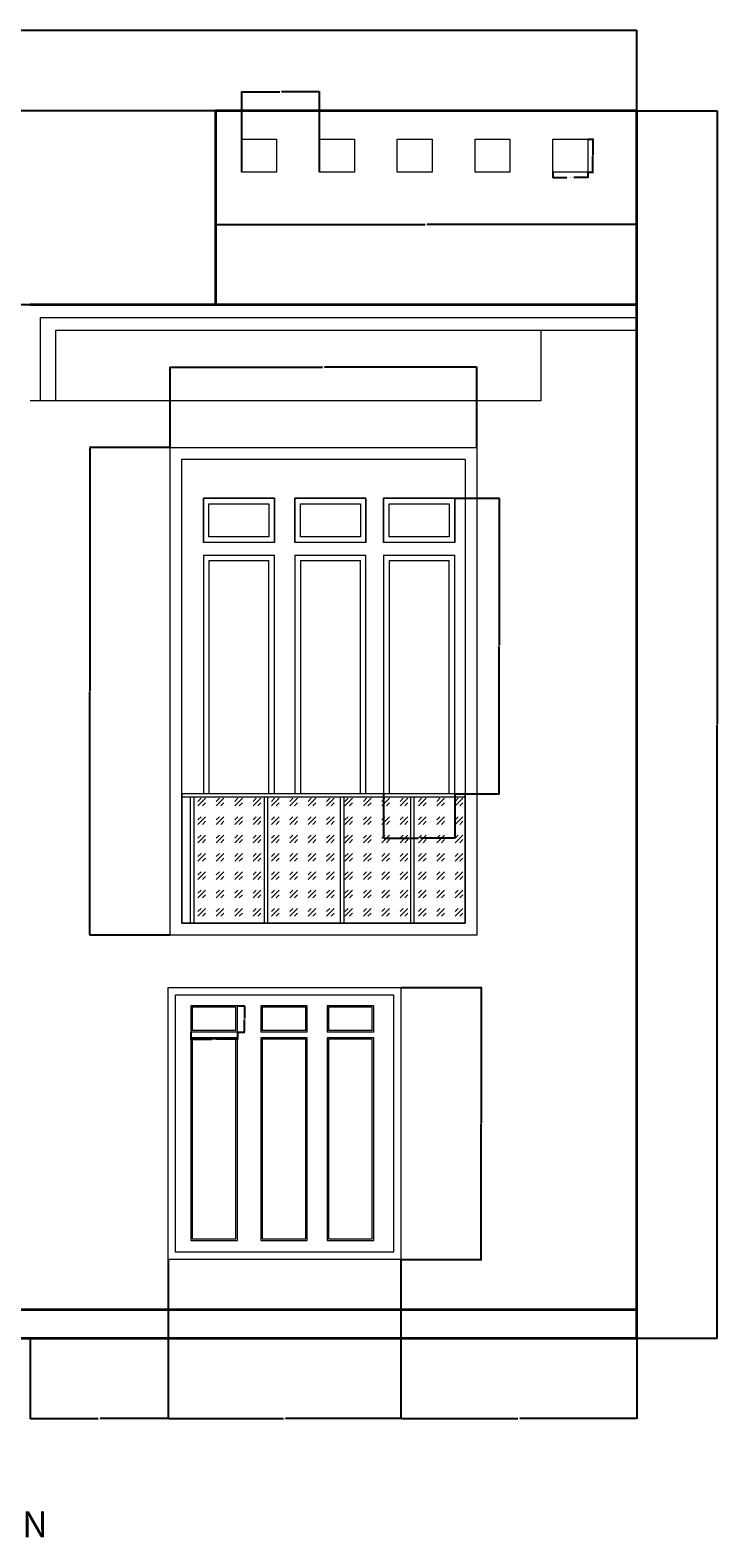
# Model space of a CAD drawing. Units: inches. Extents: x 1741 to 3812, y 9290 to 10023.
# Tile 5 of 5: x 3495 to 3812, y 9327 to 10023. Entities that reach past the tile are written whole.
import ezdxf

# ---------------------------------------------------------------- set-up
doc = ezdxf.new("R2010")
doc.units = ezdxf.units.IN
doc.header["$MEASUREMENT"] = 0
for name, color, linetype, lineweight in [('A-ANNO-DIMS', 2, 'Continuous', 18), ('A-ANNO-TEXT', 7, 'Continuous', 25), ('A-ELEV', 7, 'Continuous', 35), ('A-ELEV-RAIL', 3, 'Continuous', 18), ('A-ELEV-TRIM', 9, 'Continuous', 18), ('A-GLAZ-ELEV', 4, 'Continuous', 18), ('A-GLAZ-PATT', 8, 'Continuous', 13)]:
    doc.layers.add(name, color=color, linetype=linetype, lineweight=lineweight)
doc.styles.get("Standard").update_dxf_attribs({"font": 'arial.ttf'})
doc.dimstyles.get("Standard").update_dxf_attribs({"dimtxt": 0.18, "dimasz": 0.18, "dimexe": 0.18, "dimexo": 0.0625, "dimgap": 0.09, "dimtad": 0, "dimtih": 1, "dimtoh": 1, "dimdec": 4, "dimzin": 0, "dimdsep": 46, "dimtxsty": 'Standard', "dimcen": 0.09, "dimadec": 0, "dimazin": 0, "dimtfac": 1, "dimtdec": 4, "dimtofl": 0, "dimtmove": 0, "dimatfit": 3, "dimfxl": 1, "dimtolj": 1, "dimtzin": 0, "dimarcsym": 0})

# ---------------------------------------------------------------- blocks, each defined once
blk = doc.blocks.new('GLAZ-TRANSOM-LIGHT')
for p, q in [((0, 12.07), (0, 0)), ((21.51, 12.07), (0, 12.07)), ((0.66, 11.41), (0.66, 0.66)), ((20.85, 11.41), (0.66, 11.41)), ((20.85, 0.66), (20.85, 11.41)), ((21.51, 0), (21.51, 12.07)), ((20.85, 0.66), (0.66, 0.66)), ((21.51, 0), (0, 0))]:
    blk.add_line(p, q)
blk = doc.blocks.new('GLAZ-TALL-LIGHT-WITH-TRANSOM')
for p, q in [((0, 110.25), (32.83, 110.25)), ((2.6, 107.65), (30.23, 107.65))]:
    blk.add_line(p, q)
for points in [[(0, 136.49), (32.83, 136.49), (32.83, 116), (0, 116)], [(2.6, 133.89), (30.23, 133.89), (30.23, 118.6), (2.6, 118.6)]]:
    blk.add_lwpolyline(points, close=True)
for points in [[(32.83, 116), (32.83, 136.49), (0, 136.49), (0, 116)], [(0, 110.25), (0, 0)], [(2.6, 107.65), (2.6, 0)], [(30.23, 0), (30.23, 107.65)], [(32.83, 0), (32.83, 110.25)]]:
    blk.add_lwpolyline(points)
blk = doc.blocks.new('PARAPET-SQUARE-REVEAL')
blk.add_lwpolyline([(0, 15.35), (16.08, 15.35), (16.08, 0), (0, 0)], close=True)
blk = doc.blocks.new('*D17')
at = {"layer": 'A-ANNO-DIMS', "color": 0, "lineweight": -2, "transparency": 16777216}
for p, q in [((3569, 9560.3), (3569, 9556.96)), ((3590.51, 9560.3), (3590.51, 9556.96)), ((3569.18, 9557.14), (3578.56, 9557.14)), ((3590.33, 9557.14), (3580.95, 9557.14))]:
    blk.add_line(p, q, dxfattribs=at)
at = {"layer": 'A-ANNO-DIMS', "color": 0, "transparency": 16777216}
for points in [[(3569.18, 9557.17), (3569.18, 9557.11), (3569, 9557.14)], [(3590.33, 9557.17), (3590.33, 9557.11), (3590.51, 9557.14)]]:
    blk.add_solid(points, dxfattribs=at)
at = {"layer": 'Defpoints', "color": 0, "transparency": 16777216}
for p in [(3569, 9560.37), (3590.51, 9560.37), (3590.51, 9557.14)]:
    blk.add_point(p, dxfattribs=at)
at = {"layer": 'A-ANNO-DIMS', "color": 0, "transparency": 16777216, "insert": (3579.76, 9557.14), "char_height": 0.18, "attachment_point": 5}
blk.add_mtext('\\A1;TRANSOM 22 TYP.', dxfattribs=at)
blk = doc.blocks.new('*D18')
at = {"layer": 'A-ANNO-DIMS', "color": 0, "lineweight": -2, "transparency": 16777216}
for p, q in [((3590.58, 9572.44), (3593.92, 9572.44)), ((3593.74, 9572.26), (3593.74, 9566.58)), ((3593.74, 9560.55), (3593.74, 9566.22)), ((3590.58, 9560.37), (3593.92, 9560.37))]:
    blk.add_line(p, q, dxfattribs=at)
at = {"layer": 'A-ANNO-DIMS', "color": 0, "transparency": 16777216}
for points in [[(3593.71, 9572.26), (3593.77, 9572.26), (3593.74, 9572.44)], [(3593.71, 9560.55), (3593.77, 9560.55), (3593.74, 9560.37)]]:
    blk.add_solid(points, dxfattribs=at)
at = {"layer": 'Defpoints', "color": 0, "transparency": 16777216}
for p in [(3590.51, 9572.44), (3593.74, 9572.44), (3590.51, 9560.37)]:
    blk.add_point(p, dxfattribs=at)
at = {"layer": 'A-ANNO-DIMS', "color": 0, "transparency": 16777216, "insert": (3593.74, 9566.4), "char_height": 0.18, "attachment_point": 5}
blk.add_mtext('\\A1;12 TYP.', dxfattribs=at)
blk = doc.blocks.new('*D21')
at = {"layer": 'A-ANNO-DIMS', "color": 0, "lineweight": -2, "transparency": 16777216}
for p, q in [((3736.18, 9957.25), (3736.18, 9954.72)), ((3736.36, 9954.9), (3742.54, 9954.9)), ((3752.08, 9954.9), (3745.89, 9954.9)), ((3752.26, 9957.25), (3752.26, 9954.72))]:
    blk.add_line(p, q, dxfattribs=at)
at = {"layer": 'A-ANNO-DIMS', "color": 0, "transparency": 16777216}
for points in [[(3736.36, 9954.93), (3736.36, 9954.87), (3736.18, 9954.9)], [(3752.08, 9954.93), (3752.08, 9954.87), (3752.26, 9954.9)]]:
    blk.add_solid(points, dxfattribs=at)
at = {"layer": 'Defpoints', "color": 0, "transparency": 16777216}
for p in [(3736.18, 9957.31), (3752.26, 9957.31), (3752.26, 9954.9)]:
    blk.add_point(p, dxfattribs=at)
at = {"layer": 'A-ANNO-DIMS', "color": 0, "transparency": 16777216, "insert": (3744.22, 9954.9), "char_height": 0.18, "attachment_point": 5}
blk.add_mtext('\\A1;PARAPET REVEAL 16 TYP.', dxfattribs=at)
blk = doc.blocks.new('*D22')
at = {"layer": 'A-ANNO-DIMS', "color": 0, "lineweight": -2, "transparency": 16777216}
for p, q in [((3752.32, 9972.66), (3754.85, 9972.66)), ((3754.67, 9972.48), (3754.67, 9965.17)), ((3754.67, 9957.49), (3754.67, 9964.81)), ((3752.32, 9957.31), (3754.85, 9957.31))]:
    blk.add_line(p, q, dxfattribs=at)
at = {"layer": 'A-ANNO-DIMS', "color": 0, "transparency": 16777216}
for points in [[(3754.64, 9972.48), (3754.7, 9972.48), (3754.67, 9972.66)], [(3754.64, 9957.49), (3754.7, 9957.49), (3754.67, 9957.31)]]:
    blk.add_solid(points, dxfattribs=at)
at = {"layer": 'Defpoints', "color": 0, "transparency": 16777216}
for p in [(3752.26, 9972.66), (3754.67, 9972.66), (3752.26, 9957.31)]:
    blk.add_point(p, dxfattribs=at)
at = {"layer": 'A-ANNO-DIMS', "color": 0, "transparency": 16777216, "insert": (3754.67, 9964.99), "char_height": 0.18, "attachment_point": 5}
blk.add_mtext('\\A1;15 TYP.', dxfattribs=at)
blk = doc.blocks.new('*D27')
at = {"layer": 'A-ANNO-DIMS', "color": 0, "lineweight": -2, "transparency": 16777216}
for p, q in [((3690.93, 9806.85), (3711.52, 9806.85)), ((3711.34, 9806.67), (3711.34, 9738.79)), ((3711.34, 9670.54), (3711.34, 9738.42)), ((3690.93, 9670.36), (3711.52, 9670.36))]:
    blk.add_line(p, q, dxfattribs=at)
at = {"layer": 'A-ANNO-DIMS', "color": 0, "transparency": 16777216}
for points in [[(3711.31, 9806.67), (3711.37, 9806.67), (3711.34, 9806.85)], [(3711.31, 9670.54), (3711.37, 9670.54), (3711.34, 9670.36)]]:
    blk.add_solid(points, dxfattribs=at)
at = {"layer": 'Defpoints', "color": 0, "transparency": 16777216}
for p in [(3690.87, 9806.85), (3711.34, 9806.85), (3690.87, 9670.36)]:
    blk.add_point(p, dxfattribs=at)
at = {"layer": 'A-ANNO-DIMS', "color": 0, "transparency": 16777216, "insert": (3711.34, 9738.61), "char_height": 0.18, "attachment_point": 5}
blk.add_mtext('\\A1;TALL LIGHT 136 TYP.', dxfattribs=at)
blk = doc.blocks.new('*D28')
at = {"layer": 'A-ANNO-DIMS', "color": 0, "lineweight": -2, "transparency": 16777216}
for p, q in [((3658.04, 9670.3), (3658.04, 9649.71)), ((3690.87, 9670.3), (3690.87, 9649.71)), ((3658.22, 9649.89), (3673.93, 9649.89)), ((3690.69, 9649.89), (3674.98, 9649.89))]:
    blk.add_line(p, q, dxfattribs=at)
at = {"layer": 'A-ANNO-DIMS', "color": 0, "transparency": 16777216}
for points in [[(3658.22, 9649.92), (3658.22, 9649.86), (3658.04, 9649.89)], [(3690.69, 9649.92), (3690.69, 9649.86), (3690.87, 9649.89)]]:
    blk.add_solid(points, dxfattribs=at)
at = {"layer": 'Defpoints', "color": 0, "transparency": 16777216}
for p in [(3658.04, 9670.36), (3690.87, 9670.36), (3690.87, 9649.89)]:
    blk.add_point(p, dxfattribs=at)
at = {"layer": 'A-ANNO-DIMS', "color": 0, "transparency": 16777216, "insert": (3674.45, 9649.89), "char_height": 0.18, "attachment_point": 5}
blk.add_mtext('\\A1;33 TYP.', dxfattribs=at)
blk = doc.blocks.new('*D77')
at = {"layer": 'A-ANNO-DIMS', "color": 0, "lineweight": -2, "transparency": 16777216}
for p, q in [((3045.51, 9826.55), (3045.51, 10022.94)), ((3045.69, 10022.76), (3409.82, 10022.76)), ((3774.74, 10022.76), (3410.61, 10022.76)), ((3774.92, 9985.72), (3774.92, 10022.94))]:
    blk.add_line(p, q, dxfattribs=at)
at = {"layer": 'A-ANNO-DIMS', "color": 0, "transparency": 16777216}
for points in [[(3045.69, 10022.79), (3045.69, 10022.73), (3045.51, 10022.76)], [(3774.74, 10022.79), (3774.74, 10022.73), (3774.92, 10022.76)]]:
    blk.add_solid(points, dxfattribs=at)
at = {"layer": 'Defpoints', "color": 0, "transparency": 16777216}
for p in [(3774.92, 10022.76), (3774.92, 9985.66), (3045.51, 9826.49)]:
    blk.add_point(p, dxfattribs=at)
at = {"layer": 'A-ANNO-DIMS', "color": 0, "transparency": 16777216, "insert": (3410.21, 10022.76), "char_height": 0.18, "attachment_point": 5}
blk.add_mtext('\\A1;729.4', dxfattribs=at)
blk = doc.blocks.new('*D78')
at = {"layer": 'A-ANNO-DIMS', "color": 0, "lineweight": -2, "transparency": 16777216}
for p, q in [((3774.98, 9985.66), (3812.2, 9985.66)), ((3812.02, 9985.48), (3812.02, 9702.54)), ((3812.02, 9419.24), (3812.02, 9702.18)), ((3774.98, 9419.06), (3812.2, 9419.06))]:
    blk.add_line(p, q, dxfattribs=at)
at = {"layer": 'A-ANNO-DIMS', "color": 0, "transparency": 16777216}
for points in [[(3811.99, 9985.48), (3812.05, 9985.48), (3812.02, 9985.66)], [(3811.99, 9419.24), (3812.05, 9419.24), (3812.02, 9419.06)]]:
    blk.add_solid(points, dxfattribs=at)
at = {"layer": 'Defpoints', "color": 0, "transparency": 16777216}
for p in [(3774.92, 9985.66), (3812.02, 9985.66), (3774.92, 9419.06)]:
    blk.add_point(p, dxfattribs=at)
at = {"layer": 'A-ANNO-DIMS', "color": 0, "transparency": 16777216, "insert": (3812.02, 9702.36), "char_height": 0.18, "attachment_point": 5}
blk.add_mtext('\\A1;566.6', dxfattribs=at)
blk = doc.blocks.new('*D84')
at = {"layer": 'A-ANNO-DIMS', "color": 0, "lineweight": -2, "transparency": 16777216}
for p, q in [((3558.58, 9455.29), (3558.58, 9381.78)), ((3494.85, 9419), (3494.85, 9381.78)), ((3495.03, 9381.96), (3526.32, 9381.96)), ((3558.4, 9381.96), (3527.11, 9381.96))]:
    blk.add_line(p, q, dxfattribs=at)
at = {"layer": 'A-ANNO-DIMS', "color": 0, "transparency": 16777216}
for points in [[(3495.03, 9381.99), (3495.03, 9381.93), (3494.85, 9381.96)], [(3558.4, 9381.99), (3558.4, 9381.93), (3558.58, 9381.96)]]:
    blk.add_solid(points, dxfattribs=at)
at = {"layer": 'Defpoints', "color": 0, "transparency": 16777216}
for p in [(3558.58, 9455.35), (3494.85, 9419.06), (3558.58, 9381.96)]:
    blk.add_point(p, dxfattribs=at)
at = {"layer": 'A-ANNO-DIMS', "color": 0, "transparency": 16777216, "insert": (3526.72, 9381.96), "char_height": 0.18, "attachment_point": 5}
blk.add_mtext('\\A1;63.74', dxfattribs=at)
blk = doc.blocks.new('*D85')
at = {"layer": 'A-ANNO-DIMS', "color": 0, "lineweight": -2, "transparency": 16777216}
for p, q in [((3558.58, 9455.29), (3558.58, 9381.78)), ((3666.03, 9455.29), (3666.03, 9381.78)), ((3558.76, 9381.96), (3611.85, 9381.96)), ((3665.85, 9381.96), (3612.76, 9381.96))]:
    blk.add_line(p, q, dxfattribs=at)
at = {"layer": 'A-ANNO-DIMS', "color": 0, "transparency": 16777216}
for points in [[(3558.76, 9381.99), (3558.76, 9381.93), (3558.58, 9381.96)], [(3665.85, 9381.99), (3665.85, 9381.93), (3666.03, 9381.96)]]:
    blk.add_solid(points, dxfattribs=at)
at = {"layer": 'Defpoints', "color": 0, "transparency": 16777216}
for p in [(3558.58, 9455.35), (3666.03, 9455.35), (3666.03, 9381.96)]:
    blk.add_point(p, dxfattribs=at)
at = {"layer": 'A-ANNO-DIMS', "color": 0, "transparency": 16777216, "insert": (3612.31, 9381.96), "char_height": 0.18, "attachment_point": 5}
blk.add_mtext('\\A1;107.44', dxfattribs=at)
blk = doc.blocks.new('*D86')
at = {"layer": 'A-ANNO-DIMS', "color": 0, "lineweight": -2, "transparency": 16777216}
for p, q in [((3666.03, 9455.29), (3666.03, 9381.78)), ((3774.92, 9419), (3774.92, 9381.78)), ((3666.21, 9381.96), (3720.02, 9381.96)), ((3774.74, 9381.96), (3720.93, 9381.96))]:
    blk.add_line(p, q, dxfattribs=at)
at = {"layer": 'A-ANNO-DIMS', "color": 0, "transparency": 16777216}
for points in [[(3666.21, 9381.99), (3666.21, 9381.93), (3666.03, 9381.96)], [(3774.74, 9381.99), (3774.74, 9381.93), (3774.92, 9381.96)]]:
    blk.add_solid(points, dxfattribs=at)
at = {"layer": 'Defpoints', "color": 0, "transparency": 16777216}
for p in [(3666.03, 9455.35), (3774.92, 9419.06), (3774.92, 9381.96)]:
    blk.add_point(p, dxfattribs=at)
at = {"layer": 'A-ANNO-DIMS', "color": 0, "transparency": 16777216, "insert": (3720.47, 9381.96), "char_height": 0.18, "attachment_point": 5}
blk.add_mtext('\\A1;108.89', dxfattribs=at)
blk = doc.blocks.new('*D90')
at = {"layer": 'A-ANNO-DIMS', "color": 0, "lineweight": -2, "transparency": 16777216}
for p, q in [((3494.79, 9896.18), (3008.23, 9896.18)), ((3008.41, 9896), (3008.41, 9876.75)), ((3008.41, 9857.14), (3008.41, 9876.39)), ((3130.86, 9856.96), (3008.23, 9856.96))]:
    blk.add_line(p, q, dxfattribs=at)
at = {"layer": 'A-ANNO-DIMS', "color": 0, "transparency": 16777216}
for points in [[(3008.38, 9896), (3008.44, 9896), (3008.41, 9896.18)], [(3008.38, 9857.14), (3008.44, 9857.14), (3008.41, 9856.96)]]:
    blk.add_solid(points, dxfattribs=at)
at = {"layer": 'Defpoints', "color": 0, "transparency": 16777216}
for p in [(3008.41, 9896.18), (3494.85, 9896.18), (3130.92, 9856.96)]:
    blk.add_point(p, dxfattribs=at)
at = {"layer": 'A-ANNO-DIMS', "color": 0, "transparency": 16777216, "insert": (3008.41, 9876.57), "char_height": 0.18, "attachment_point": 5}
blk.add_mtext('\\A1;39.22', dxfattribs=at)
blk = doc.blocks.new('*D91')
at = {"layer": 'A-ANNO-DIMS', "color": 0, "lineweight": -2, "transparency": 16777216}
for p, q in [((3580.43, 9985.66), (3008.23, 9985.66)), ((3008.41, 9985.48), (3008.41, 9941.1)), ((3008.41, 9896.36), (3008.41, 9940.74)), ((3494.79, 9896.18), (3008.23, 9896.18))]:
    blk.add_line(p, q, dxfattribs=at)
at = {"layer": 'A-ANNO-DIMS', "color": 0, "transparency": 16777216}
for points in [[(3008.38, 9985.48), (3008.44, 9985.48), (3008.41, 9985.66)], [(3008.38, 9896.36), (3008.44, 9896.36), (3008.41, 9896.18)]]:
    blk.add_solid(points, dxfattribs=at)
at = {"layer": 'Defpoints', "color": 0, "transparency": 16777216}
for p in [(3008.41, 9985.66), (3580.49, 9985.66), (3494.85, 9896.18)]:
    blk.add_point(p, dxfattribs=at)
at = {"layer": 'A-ANNO-DIMS', "color": 0, "transparency": 16777216, "insert": (3008.41, 9940.92), "char_height": 0.18, "attachment_point": 5}
blk.add_mtext('\\A1;89.48', dxfattribs=at)
blk = doc.blocks.new('*D92')
at = {"layer": 'A-ANNO-DIMS', "color": 0, "lineweight": -2, "transparency": 16777216}
for p, q in [((3580.49, 9896.24), (3580.49, 9933.46)), ((3580.67, 9933.28), (3677.25, 9933.28)), ((3774.74, 9933.28), (3678.16, 9933.28)), ((3774.92, 9896.24), (3774.92, 9933.46))]:
    blk.add_line(p, q, dxfattribs=at)
at = {"layer": 'A-ANNO-DIMS', "color": 0, "transparency": 16777216}
for points in [[(3580.67, 9933.31), (3580.67, 9933.25), (3580.49, 9933.28)], [(3774.74, 9933.31), (3774.74, 9933.25), (3774.92, 9933.28)]]:
    blk.add_solid(points, dxfattribs=at)
at = {"layer": 'Defpoints', "color": 0, "transparency": 16777216}
for p in [(3774.92, 9933.28), (3580.49, 9896.18), (3774.92, 9896.18)]:
    blk.add_point(p, dxfattribs=at)
at = {"layer": 'A-ANNO-DIMS', "color": 0, "transparency": 16777216, "insert": (3677.7, 9933.28), "char_height": 0.18, "attachment_point": 5}
blk.add_mtext('\\A1;194.43', dxfattribs=at)
blk = doc.blocks.new('*D93')
at = {"layer": 'A-ANNO-DIMS', "color": 0, "lineweight": -2, "transparency": 16777216}
for p, q in [((3666.09, 9580.95), (3703.31, 9580.95)), ((3703.13, 9580.77), (3703.13, 9518.33)), ((3703.13, 9455.53), (3703.13, 9517.97)), ((3666.09, 9455.35), (3703.31, 9455.35))]:
    blk.add_line(p, q, dxfattribs=at)
at = {"layer": 'A-ANNO-DIMS', "color": 0, "transparency": 16777216}
for points in [[(3703.1, 9580.77), (3703.16, 9580.77), (3703.13, 9580.95)], [(3703.1, 9455.53), (3703.16, 9455.53), (3703.13, 9455.35)]]:
    blk.add_solid(points, dxfattribs=at)
at = {"layer": 'Defpoints', "color": 0, "transparency": 16777216}
for p in [(3666.03, 9580.95), (3666.03, 9455.35), (3703.13, 9455.35)]:
    blk.add_point(p, dxfattribs=at)
at = {"layer": 'A-ANNO-DIMS', "color": 0, "transparency": 16777216, "insert": (3703.13, 9518.15), "char_height": 0.18, "attachment_point": 5}
blk.add_mtext('\\A1;125.6', dxfattribs=at)
blk = doc.blocks.new('*D96')
at = {"layer": 'A-ANNO-DIMS', "color": 0, "lineweight": -2, "transparency": 16777216}
for p, q in [((3559.45, 9830.28), (3522.24, 9830.28)), ((3522.42, 9830.1), (3522.42, 9717.89)), ((3522.42, 9605.32), (3522.42, 9717.52)), ((3559.45, 9605.14), (3522.24, 9605.14))]:
    blk.add_line(p, q, dxfattribs=at)
at = {"layer": 'A-ANNO-DIMS', "color": 0, "transparency": 16777216}
for points in [[(3522.39, 9830.1), (3522.45, 9830.1), (3522.42, 9830.28)], [(3522.39, 9605.32), (3522.45, 9605.32), (3522.42, 9605.14)]]:
    blk.add_solid(points, dxfattribs=at)
at = {"layer": 'Defpoints', "color": 0, "transparency": 16777216}
for p in [(3522.42, 9830.28), (3559.52, 9830.28), (3559.52, 9605.14)]:
    blk.add_point(p, dxfattribs=at)
at = {"layer": 'A-ANNO-DIMS', "color": 0, "transparency": 16777216, "insert": (3522.42, 9717.71), "char_height": 0.18, "attachment_point": 5}
blk.add_mtext('\\A1;225.14', dxfattribs=at)
blk = doc.blocks.new('*D97')
at = {"layer": 'A-ANNO-DIMS', "color": 0, "lineweight": -2, "transparency": 16777216}
for p, q in [((3559.52, 9830.34), (3559.52, 9867.56)), ((3559.7, 9867.38), (3629.82, 9867.38)), ((3700.85, 9867.38), (3630.73, 9867.38)), ((3701.03, 9830.34), (3701.03, 9867.56))]:
    blk.add_line(p, q, dxfattribs=at)
at = {"layer": 'A-ANNO-DIMS', "color": 0, "transparency": 16777216}
for points in [[(3559.7, 9867.41), (3559.7, 9867.35), (3559.52, 9867.38)], [(3700.85, 9867.41), (3700.85, 9867.35), (3701.03, 9867.38)]]:
    blk.add_solid(points, dxfattribs=at)
at = {"layer": 'Defpoints', "color": 0, "transparency": 16777216}
for p in [(3701.03, 9867.38), (3559.52, 9830.28), (3701.03, 9830.28)]:
    blk.add_point(p, dxfattribs=at)
at = {"layer": 'A-ANNO-DIMS', "color": 0, "transparency": 16777216, "insert": (3630.27, 9867.38), "char_height": 0.18, "attachment_point": 5}
blk.add_mtext('\\A1;141.52', dxfattribs=at)
blk = doc.blocks.new('*D101')
at = {"layer": 'A-ANNO-DIMS', "color": 0, "lineweight": -2, "transparency": 16777216}
for p, q in [((3592.53, 9957.37), (3592.53, 9994.59)), ((3592.71, 9994.41), (3610.11, 9994.41)), ((3628.26, 9994.41), (3610.86, 9994.41)), ((3628.44, 9957.37), (3628.44, 9994.59))]:
    blk.add_line(p, q, dxfattribs=at)
at = {"layer": 'A-ANNO-DIMS', "color": 0, "transparency": 16777216}
for points in [[(3592.71, 9994.44), (3592.71, 9994.38), (3592.53, 9994.41)], [(3628.26, 9994.44), (3628.26, 9994.38), (3628.44, 9994.41)]]:
    blk.add_solid(points, dxfattribs=at)
at = {"layer": 'Defpoints', "color": 0, "transparency": 16777216}
for p in [(3628.44, 9994.41), (3592.53, 9957.31), (3628.44, 9957.31)]:
    blk.add_point(p, dxfattribs=at)
at = {"layer": 'A-ANNO-DIMS', "color": 0, "transparency": 16777216, "insert": (3610.48, 9994.41), "char_height": 0.18, "attachment_point": 5}
blk.add_mtext('\\A1;35.91', dxfattribs=at)

msp = doc.modelspace()

# ---------------------------------------------------------------- hatches: boundary and pattern name
at = {"layer": 'A-GLAZ-PATT'}
h = msp.add_hatch(dxfattribs=at)
h.set_pattern_fill('GOST_GLASS', color=256)
h.set_pattern_definition([(45, (0, 0), (8.4852814, 0), [5, -7]), (45, (2.1213, 0), (8.4852814, 0), [2, -10]), (45, (0, 2.1213), (8.4852814, 0), [2, -10])])
h.paths.add_polyline_path([(3602.9568, 9668.8926), (3570.4425, 9668.8926), (3570.4425, 9610.5506), (3602.9568, 9610.5506)])
h.paths.add_polyline_path([(3638.1419, 9668.8926), (3604.4755, 9668.8926), (3604.4755, 9610.5506), (3638.1419, 9610.5506)])
h.paths.add_polyline_path([(3670.5198, 9668.8926), (3639.6606, 9668.8926), (3639.6606, 9610.5506), (3670.5198, 9610.5506)])
h.paths.add_polyline_path([(3695.6162, 9668.8926), (3672.0386, 9668.8926), (3672.0386, 9610.5506), (3695.6162, 9610.5506)])

# ---------------------------------------------------------------- linework, layer by layer
at = {"layer": 'A-ELEV'}
for p, q in [((3774.9155, 9985.6625), (3580.4882, 9985.6625)), ((3580.4882, 9985.6625), (3580.4882, 9896.1797)), ((3774.9155, 9887.7993), (3774.9155, 9985.6625)), ((3774.9155, 9896.1797), (3494.8475, 9896.1797)), ((3774.9155, 9419.0599), (3774.9155, 9887.7993)), ((3130.9182, 9432.1944), (3774.9155, 9432.1944)), ((3130.9182, 9419.0599), (3774.9155, 9419.0599))]:
    msp.add_line(p, q, dxfattribs=at)
at = {"layer": 'A-ELEV-RAIL'}
msp.add_line((3564.9309, 9668.8926), (3695.6162, 9668.8926), dxfattribs=at)
for points in [[(3564.9309, 9610.5506), (3695.6162, 9610.5506), (3695.6162, 9670.3623), (3564.9309, 9670.3623)], [(3568.9238, 9668.8926), (3570.4425, 9668.8926), (3570.4425, 9610.5506), (3568.9238, 9610.5506)], [(3602.9568, 9668.8926), (3604.4755, 9668.8926), (3604.4755, 9610.5506), (3602.9568, 9610.5506)], [(3638.1419, 9668.8926), (3639.6606, 9668.8926), (3639.6606, 9610.5506), (3638.1419, 9610.5506)], [(3670.5198, 9668.8926), (3672.0386, 9668.8926), (3672.0386, 9610.5506), (3670.5198, 9610.5506)]]:
    msp.add_lwpolyline(points, close=True, dxfattribs=at)
at = {"layer": 'A-ELEV-TRIM'}
for p, q in [((3499.6507, 9851.7953), (3499.6507, 9890.3322)), ((3499.6507, 9890.3322), (3774.9155, 9890.3322)), ((3506.6417, 9851.7953), (3506.6417, 9884.4731)), ((3506.6417, 9884.4731), (3774.9155, 9884.4731)), ((3730.5782, 9884.4731), (3730.5782, 9851.7953)), ((3730.5782, 9851.7953), (3494.8475, 9851.7953))]:
    msp.add_line(p, q, dxfattribs=at)
at = {"layer": 'A-GLAZ-ELEV'}
for p, q in [((3590.515, 9557.7018), (3569.0015, 9557.7018)), ((3569.0015, 9557.7018), (3569.0015, 9464.1476)), ((3589.8533, 9557.0401), (3569.6633, 9557.0401)), ((3569.6633, 9557.0401), (3569.6633, 9464.8093)), ((3589.8533, 9464.8093), (3589.8533, 9557.0401)), ((3590.515, 9464.1476), (3590.515, 9557.7018)), ((3569.0015, 9464.1476), (3590.515, 9464.1476)), ((3569.6633, 9464.8093), (3589.8533, 9464.8093))]:
    msp.add_line(p, q, dxfattribs=at)
for points in [[(3559.5155, 9830.2772), (3701.0316, 9830.2772), (3701.0316, 9605.1352), (3559.5155, 9605.1352)], [(3564.9309, 9824.8618), (3695.6162, 9824.8618), (3695.6162, 9610.5506), (3564.9309, 9610.5506)], [(3558.5845, 9580.9464), (3666.029, 9580.9464), (3666.029, 9455.3507), (3558.5845, 9455.3507)], [(3562.0207, 9577.5102), (3662.5927, 9577.5102), (3662.5927, 9458.7869), (3562.0207, 9458.7869)], [(3601.2718, 9464.1476), (3622.7852, 9464.1476), (3622.7852, 9557.7018), (3601.2718, 9557.7018)], [(3601.9335, 9464.8093), (3622.1235, 9464.8093), (3622.1235, 9557.0401), (3601.9335, 9557.0401)], [(3631.9483, 9464.1476), (3653.4618, 9464.1476), (3653.4618, 9557.7018), (3631.9483, 9557.7018)], [(3632.6101, 9464.8093), (3652.8, 9464.8093), (3652.8, 9557.0401), (3632.6101, 9557.0401)]]:
    msp.add_lwpolyline(points, close=True, dxfattribs=at)

# ---------------------------------------------------------------- block references
at = {"layer": 'A-ELEV-TRIM'}
for p in [(3592.527, 9957.31), (3628.4394, 9957.31), (3664.3517, 9957.31), (3700.2641, 9957.31), (3736.1764, 9957.31)]:
    msp.add_blockref('PARAPET-SQUARE-REVEAL', p, dxfattribs=at)
at = {"layer": 'A-GLAZ-ELEV'}
for name, p in [('GLAZ-TALL-LIGHT-WITH-TRANSOM', (3574.798, 9670.362)), ('GLAZ-TALL-LIGHT-WITH-TRANSOM', (3617.0476, 9670.362)), ('GLAZ-TALL-LIGHT-WITH-TRANSOM', (3658.0403, 9670.362)), ('GLAZ-TRANSOM-LIGHT', (3569.002, 9560.367)), ('GLAZ-TRANSOM-LIGHT', (3601.2722, 9560.367)), ('GLAZ-TRANSOM-LIGHT', (3631.9488, 9560.367))]:
    msp.add_blockref(name, p, dxfattribs=at)

# ---------------------------------------------------------------- texts
at = {"layer": 'A-ANNO-TEXT'}
msp.add_text('FRONT ELEVATION', height=12, dxfattribs=at).set_placement((3359.9256, 9327.0309))

# ---------------------------------------------------------------- dimensions: what is measured, and where the dimension line sits
at = {"layer": 'A-ANNO-DIMS'}
for base, p1, p2, override, picture, middle in [((3774.9155, 10022.7625), (3045.5138, 9826.4899), (3774.9155, 9985.6625), {"dimdec": 1, "dimlfac": 1, "dimrnd": 0, "dimzin": 0, "dimdsep": 46, "dimlunit": 2}, '*D77', (3410.2146, 10022.7625)), ((3628.4395, 9994.41), (3592.5271, 9957.31), (3628.4395, 9957.31), {"dimdec": 2, "dimlfac": 1, "dimrnd": 0, "dimzin": 0, "dimdsep": 46, "dimlunit": 2}, '*D101', (3610.4833, 9994.41)), ((3774.9155, 9933.2797), (3580.4882, 9896.1797), (3774.9155, 9896.1797), {"dimdec": 2, "dimlfac": 1, "dimrnd": 0, "dimzin": 0, "dimdsep": 46, "dimlunit": 2}, '*D92', (3677.7018, 9933.2797)), ((3701.0316, 9867.3772), (3559.5155, 9830.2772), (3701.0316, 9830.2772), {"dimdec": 2, "dimlfac": 1, "dimrnd": 0, "dimzin": 0, "dimdsep": 46, "dimlunit": 2}, '*D97', (3630.2735, 9867.3772)), ((3558.5845, 9381.9599), (3494.8475, 9419.0599), (3558.5845, 9455.3507), {"dimdec": 2, "dimlfac": 1, "dimrnd": 0, "dimzin": 0, "dimdsep": 46, "dimlunit": 2}, '*D84', (3526.716, 9381.9599)), ((3666.029, 9381.9599), (3558.5845, 9455.3507), (3666.029, 9455.3507), {"dimdec": 2, "dimlfac": 1, "dimrnd": 0, "dimzin": 0, "dimdsep": 46, "dimlunit": 2}, '*D85', (3612.3067, 9381.9599)), ((3774.9155, 9381.9599), (3666.029, 9455.3507), (3774.9155, 9419.0599), {"dimdec": 2, "dimlfac": 1, "dimrnd": 0, "dimzin": 0, "dimdsep": 46, "dimlunit": 2}, '*D86', (3720.4722, 9381.9599))]:
    dim = msp.add_linear_dim(base=base, p1=p1, p2=p2, dimstyle='Standard', override=override, dxfattribs=at)
    dim.commit()
    dim.dimension.update_dxf_attribs({"geometry": picture, "text_midpoint": middle})
for base, p1, p2, angle, override, picture, middle in [((3008.4138, 9985.6625), (3494.8475, 9896.1797), (3580.4882, 9985.6625), 90, {"dimdec": 2, "dimlfac": 1, "dimrnd": 0, "dimzin": 0, "dimdsep": 46, "dimlunit": 2}, '*D91', (3008.4138, 9940.9211)), ((3812.0155, 9985.6625), (3774.9155, 9419.0599), (3774.9155, 9985.6625), 90, {"dimdec": 1, "dimlfac": 1, "dimrnd": 0, "dimzin": 0, "dimdsep": 46, "dimlunit": 2}, '*D78', (3812.0155, 9702.3612)), ((3008.4138, 9896.1797), (3130.9182, 9856.9629), (3494.8475, 9896.1797), 90, {"dimdec": 2, "dimlfac": 1, "dimrnd": 0, "dimzin": 0, "dimdsep": 46, "dimlunit": 2}, '*D90', (3008.4138, 9876.5713)), ((3522.4155, 9830.2772), (3559.5155, 9605.1352), (3559.5155, 9830.2772), 90, {"dimdec": 2, "dimlfac": 1, "dimrnd": 0, "dimzin": 0, "dimdsep": 46, "dimlunit": 2}, '*D96', (3522.4155, 9717.7062)), ((3703.129, 9455.3507), (3666.029, 9580.9464), (3666.029, 9455.3507), 270, {"dimdec": 1, "dimlfac": 1, "dimrnd": 0, "dimzin": 0, "dimdsep": 46, "dimlunit": 2}, '*D93', (3703.129, 9518.1485))]:
    dim = msp.add_linear_dim(base=base, p1=p1, p2=p2, angle=angle, dimstyle='Standard', override=override, dxfattribs=at)
    dim.commit()
    dim.dimension.update_dxf_attribs({"geometry": picture, "text_midpoint": middle})
for base, p1, p2, text, picture, middle in [((3754.6688, 9972.6641), (3752.2567, 9957.31), (3752.2567, 9972.6641), '<> TYP.', '*D22', (3754.6688, 9964.987)), ((3711.3412, 9806.8491), (3690.8682, 9670.3623), (3690.8682, 9806.8491), 'TALL LIGHT <> TYP.', '*D27', (3711.3412, 9738.6057)), ((3593.742, 9572.4354), (3590.515, 9560.3668), (3590.515, 9572.4354), '<> TYP.', '*D18', (3593.742, 9566.4011))]:
    dim = msp.add_linear_dim(base=base, p1=p1, p2=p2, angle=90, text=text, dimstyle='Standard', override={"dimdec": 0, "dimlfac": 1, "dimrnd": 0, "dimzin": 0, "dimdsep": 46, "dimlunit": 2}, dxfattribs=at)
    dim.commit()
    dim.dimension.update_dxf_attribs({"geometry": picture, "text_midpoint": middle})
for base, p1, p2, text, picture, middle in [((3752.2567, 9954.898), (3736.1766, 9957.31), (3752.2567, 9957.31), 'PARAPET REVEAL <> TYP.', '*D21', (3744.2167, 9954.898)), ((3690.8682, 9649.8893), (3658.0402, 9670.3623), (3690.8682, 9670.3623), '<> TYP.', '*D28', (3674.4542, 9649.8893)), ((3590.515, 9557.1398), (3569.0015, 9560.3668), (3590.515, 9560.3668), 'TRANSOM <> TYP.', '*D17', (3579.7583, 9557.1398))]:
    dim = msp.add_linear_dim(base=base, p1=p1, p2=p2, text=text, dimstyle='Standard', override={"dimdec": 0, "dimlfac": 1, "dimrnd": 0, "dimzin": 0, "dimdsep": 46, "dimlunit": 2}, dxfattribs=at)
    dim.commit()
    dim.dimension.update_dxf_attribs({"geometry": picture, "text_midpoint": middle})

doc.saveas('drawing.dxf')
